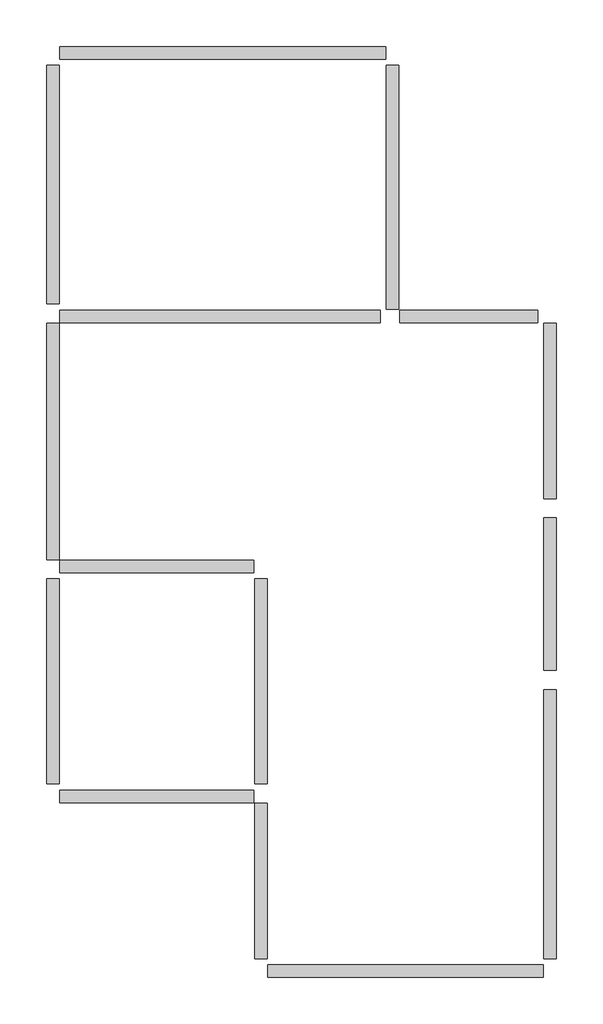
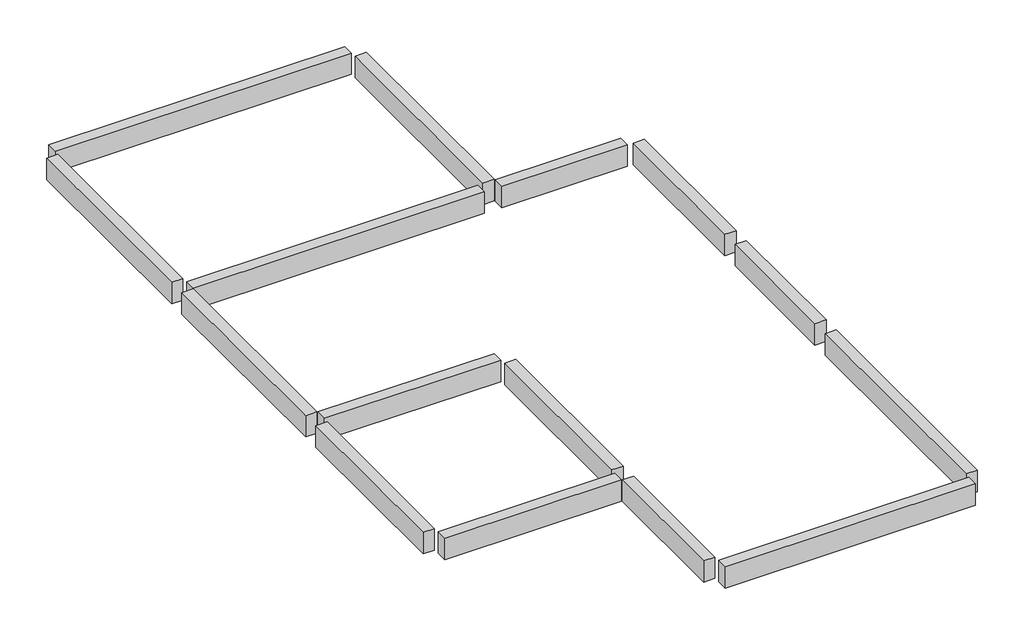
# One storey: 15 beams.
"""IFC4 building model written with IfcOpenShell, lengths in millimetres."""

from ifc_helpers import new_model, si_unit, frame, origin, place, context, project, spatial, polyline, outline, extrude, element, save

model = new_model("IFC4")

# Units and contexts
model_context = context("Model", 3, world=origin())
ifc_project = project(units=[si_unit("LENGTHUNIT", "METRE", prefix="MILLI")], contexts=[model_context])

# Site, building, storey
site = spatial("IfcSite", under=ifc_project)
building = spatial("IfcBuilding", under=site)
storey = spatial("IfcBuildingStorey", under=building, Elevation=3200.4)

# Beams
placement = place(None, origin())
element("IfcBeam", 1, ObjectType="Concrete-Rectangular Beam : 10\" x 24\"", at=placement, inside=storey, context=model_context, shape_type="SweptSolid", body=[
    extrude(outline(polyline([(-12235.0833659, 12888.2783402), (-12235.0833659, 13116.8783402), (-6266.0833659, 13116.8783402), (-6266.0833659, 12888.2783402), (-12235.0833659, 12888.2783402)])), frame((0.0, 0.0, 2743.2), z_axis=(0.0, 0.0, 1.0), x_axis=(1.0, 0.0, 0.0)), (0.0, 0.0, 1.0), 457.2),
])
element("IfcBeam", 2, ObjectType="Concrete-Rectangular Beam : 10\" x 24\"", at=placement, inside=storey, context=model_context, shape_type="SweptSolid", body=[
    extrude(outline(polyline([(-6253.3833659, 12773.9783402), (-6024.7833659, 12773.9783402), (-6024.7833659, 8303.5783402), (-6253.3833659, 8303.5783402), (-6253.3833659, 12773.9783402)])), frame((0.0, 0.0, 2743.2), z_axis=(0.0, 0.0, 1.0), x_axis=(1.0, 0.0, 0.0)), (0.0, 0.0, 1.0), 457.2),
])
element("IfcBeam", 3, ObjectType="Concrete-Rectangular Beam : 10\" x 24\"", at=placement, inside=storey, context=model_context, shape_type="SweptSolid", body=[
    extrude(outline(polyline([(-3484.7833659, 8290.8783402), (-3484.7833659, 8062.2783402), (-6012.0833659, 8062.2783402), (-6012.0833659, 8290.8783402), (-3484.7833659, 8290.8783402)])), frame((0.0, 0.0, 2743.2), z_axis=(0.0, 0.0, 1.0), x_axis=(1.0, 0.0, 0.0)), (0.0, 0.0, 1.0), 457.2),
])
element("IfcBeam", 4, ObjectType="Concrete-Rectangular Beam : 10\" x 24\"", at=placement, inside=storey, context=model_context, shape_type="SweptSolid", body=[
    extrude(outline(polyline([(-3142.0191189, 4841.8494441), (-3370.6191189, 4841.8494441), (-3370.6191189, 8049.5783402), (-3142.0191189, 8049.5783402), (-3142.0191189, 4841.8494441)])), frame((0.0, 0.0, 2743.2), z_axis=(0.0, 0.0, 1.0), x_axis=(1.0, 0.0, 0.0)), (0.0, 0.0, 1.0), 457.2),
])
element("IfcBeam", 5, ObjectType="Concrete-Rectangular Beam : 10\" x 24\"", at=placement, inside=storey, context=model_context, shape_type="SweptSolid", body=[
    extrude(outline(polyline([(-3142.0191189, 1700.3598175), (-3370.6191189, 1700.3598175), (-3370.6191189, 4486.2494441), (-3142.0191189, 4486.2494441), (-3142.0191189, 1700.3598175)])), frame((0.0, 0.0, 2743.2), z_axis=(0.0, 0.0, 1.0), x_axis=(1.0, 0.0, 0.0)), (0.0, 0.0, 1.0), 457.2),
])
element("IfcBeam", 6, ObjectType="Concrete-Rectangular Beam : 10\" x 24\"", at=placement, inside=storey, context=model_context, shape_type="SweptSolid", body=[
    extrude(outline(polyline([(-3370.6191189, 1344.7598175), (-3142.0191189, 1344.7598175), (-3142.0191189, -3583.6216598), (-3370.6191189, -3583.6216598), (-3370.6191189, 1344.7598175)])), frame((0.0, 0.0, 2743.2), z_axis=(0.0, 0.0, 1.0), x_axis=(1.0, 0.0, 0.0)), (0.0, 0.0, 1.0), 457.2),
])
element("IfcBeam", 7, ObjectType="Concrete-Rectangular Beam : 10\" x 24\"", at=placement, inside=storey, context=model_context, shape_type="SweptSolid", body=[
    extrude(outline(polyline([(-3383.3191189, -3697.9216598), (-3383.3191189, -3926.5216598), (-8425.0833659, -3926.5216598), (-8425.0833659, -3697.9216598), (-3383.3191189, -3697.9216598)])), frame((0.0, 0.0, 2743.2), z_axis=(0.0, 0.0, 1.0), x_axis=(1.0, 0.0, 0.0)), (0.0, 0.0, 1.0), 457.2),
])
element("IfcBeam", 8, ObjectType="Concrete-Rectangular Beam : 10\" x 24\"", at=placement, inside=storey, context=model_context, shape_type="SweptSolid", body=[
    extrude(outline(polyline([(-8437.7833659, -3583.6216598), (-8666.3833659, -3583.6216598), (-8666.3833659, -738.8216598), (-8437.7833659, -738.8216598), (-8437.7833659, -3583.6216598)])), frame((0.0, 0.0, 2743.2), z_axis=(0.0, 0.0, 1.0), x_axis=(1.0, 0.0, 0.0)), (0.0, 0.0, 1.0), 457.2),
])
element("IfcBeam", 9, ObjectType="Concrete-Rectangular Beam : 10\" x 24\"", at=placement, inside=storey, context=model_context, shape_type="SweptSolid", body=[
    extrude(outline(polyline([(-8666.3833659, 3369.6283402), (-8437.7833659, 3369.6283402), (-8437.7833659, -383.2216598), (-8666.3833659, -383.2216598), (-8666.3833659, 3369.6283402)])), frame((0.0, 0.0, 2743.2), z_axis=(0.0, 0.0, 1.0), x_axis=(1.0, 0.0, 0.0)), (0.0, 0.0, 1.0), 457.2),
])
element("IfcBeam", 10, ObjectType="Concrete-Rectangular Beam : 10\" x 24\"", at=placement, inside=storey, context=model_context, shape_type="SweptSolid", body=[
    extrude(outline(polyline([(-12235.0833659, 3483.9283402), (-12235.0833659, 3712.5283402), (-8679.0833659, 3712.5283402), (-8679.0833659, 3483.9283402), (-12235.0833659, 3483.9283402)])), frame((0.0, 0.0, 2743.2), z_axis=(0.0, 0.0, 1.0), x_axis=(1.0, 0.0, 0.0)), (0.0, 0.0, 1.0), 457.2),
])
element("IfcBeam", 11, ObjectType="Concrete-Rectangular Beam : 10\" x 24\"", at=placement, inside=storey, context=model_context, shape_type="SweptSolid", body=[
    extrude(outline(polyline([(-12247.7833659, -383.2216598), (-12476.3833659, -383.2216598), (-12476.3833659, 3369.6283402), (-12247.7833659, 3369.6283402), (-12247.7833659, -383.2216598)])), frame((0.0, 0.0, 2743.2), z_axis=(0.0, 0.0, 1.0), x_axis=(1.0, 0.0, 0.0)), (0.0, 0.0, 1.0), 457.2),
])
element("IfcBeam", 12, ObjectType="Concrete-Rectangular Beam : 10\" x 24\"", at=placement, inside=storey, context=model_context, shape_type="SweptSolid", body=[
    extrude(outline(polyline([(-12235.0833659, -726.1216598), (-12235.0833659, -497.5216598), (-8679.0833659, -497.5216598), (-8679.0833659, -726.1216598), (-12235.0833659, -726.1216598)])), frame((0.0, 0.0, 2743.2), z_axis=(0.0, 0.0, 1.0), x_axis=(1.0, 0.0, 0.0)), (0.0, 0.0, 1.0), 457.2),
])
element("IfcBeam", 13, ObjectType="Concrete-Rectangular Beam : 10\" x 24\"", at=placement, inside=storey, context=model_context, shape_type="SweptSolid", body=[
    extrude(outline(polyline([(-12247.7833659, 3725.2283402), (-12476.3833659, 3725.2283402), (-12476.3833659, 8049.5783402), (-12247.7833659, 8049.5783402), (-12247.7833659, 3725.2283402)])), frame((0.0, 0.0, 2743.2), z_axis=(0.0, 0.0, 1.0), x_axis=(1.0, 0.0, 0.0)), (0.0, 0.0, 1.0), 457.2),
])
element("IfcBeam", 14, ObjectType="Concrete-Rectangular Beam : 10\" x 24\"", at=placement, inside=storey, context=model_context, shape_type="SweptSolid", body=[
    extrude(outline(polyline([(-12247.7833659, 8405.1783402), (-12476.3833659, 8405.1783402), (-12476.3833659, 12773.9783402), (-12247.7833659, 12773.9783402), (-12247.7833659, 8405.1783402)])), frame((0.0, 0.0, 2743.2), z_axis=(0.0, 0.0, 1.0), x_axis=(1.0, 0.0, 0.0)), (0.0, 0.0, 1.0), 457.2),
])
element("IfcBeam", 15, ObjectType="Concrete-Rectangular Beam : 10\" x 24\"", at=placement, inside=storey, context=model_context, shape_type="SweptSolid", body=[
    extrude(outline(polyline([(-6367.6833659, 8290.8783402), (-6367.6833659, 8062.2783402), (-12235.0833659, 8062.2783402), (-12235.0833659, 8290.8783402), (-6367.6833659, 8290.8783402)])), frame((0.0, 0.0, 2743.2), z_axis=(0.0, 0.0, 1.0), x_axis=(1.0, 0.0, 0.0)), (0.0, 0.0, 1.0), 457.2),
])

save(model, "model.ifc")

# Revit data of these elements
# Type "Concrete-Rectangular Beam : 10\" x 24\""
#   Assembly Code = "B10"
#   Length [instance default] = 5' - 0"
#   b = 0' - 9"
#   h = 1' - 6"
#   Structural Material [instance default] = Concrete, Cast-in-Place gray
# Elements 1, 2, 3, 4, 5, 6, 7, 8, 9, 10, 11, 12, 13, 14, 15 (IfcBeam, "Concrete-Rectangular Beam : 10\" x 24\"")
#   Structural Material = Concrete, Cast-in-Place gray
#   Phase Created = New Construction
#   Materials on its faces: "Concrete, Cast-in-Place gray"
# Materials
#   "Concrete, Cast-in-Place gray": class "Concrete", colour RGB 192 192 192, transparency 0, Description = "Cast-in-place concrete", Cost = 0
